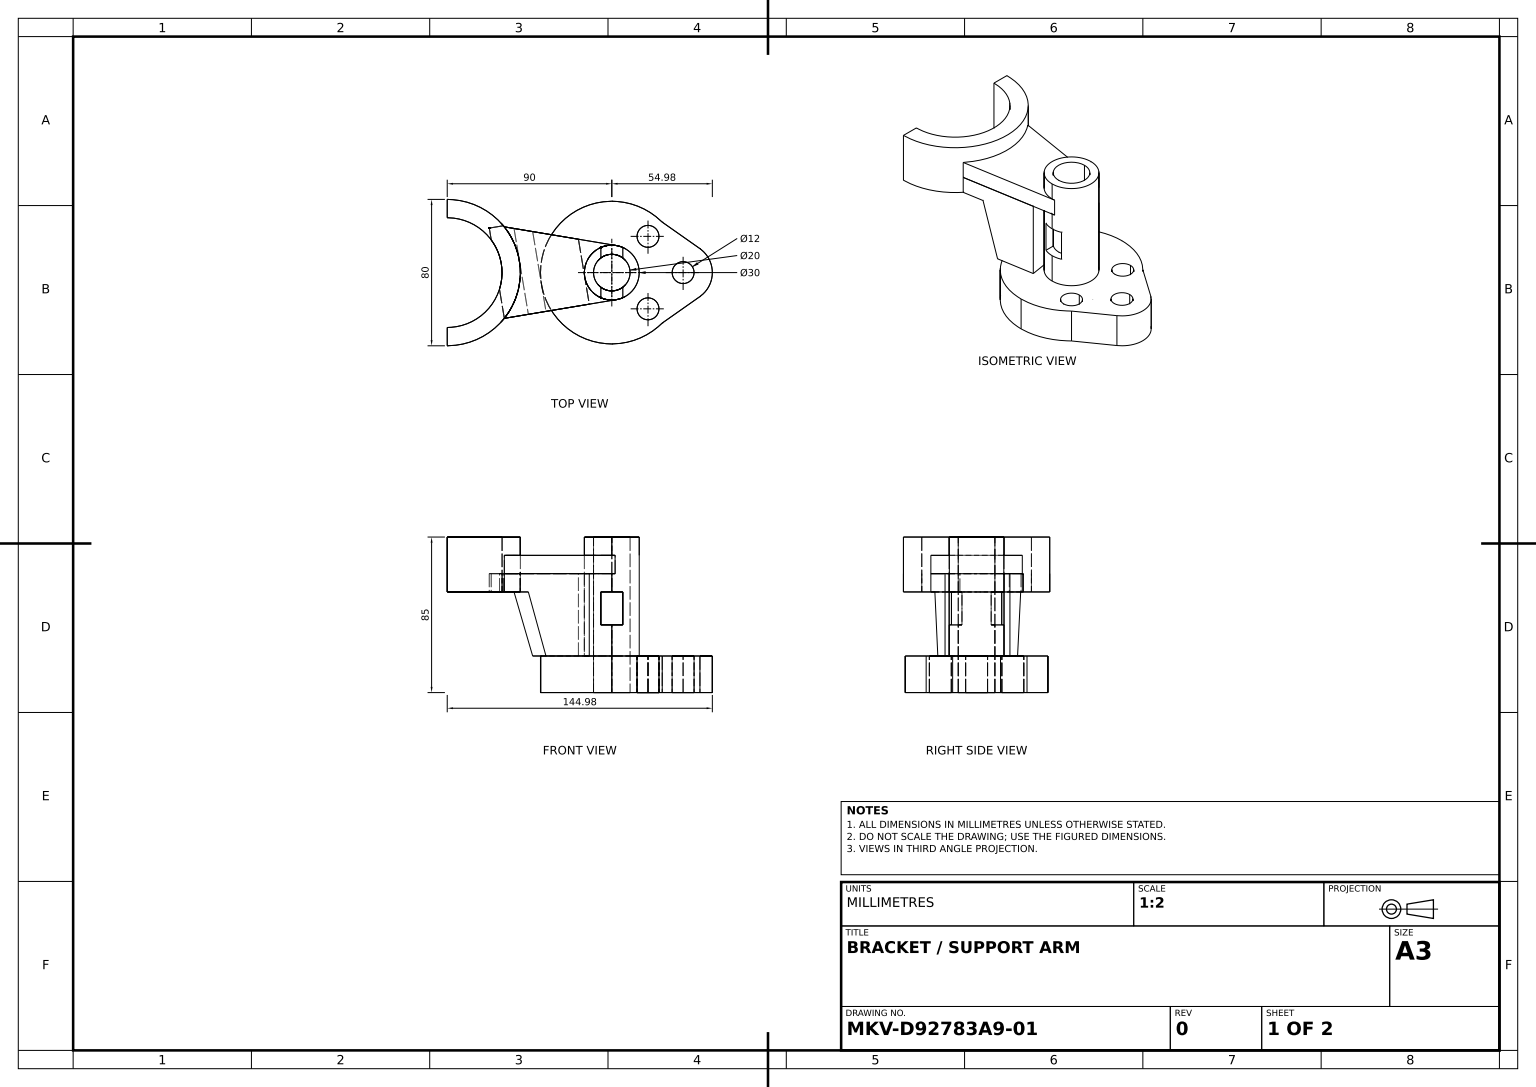
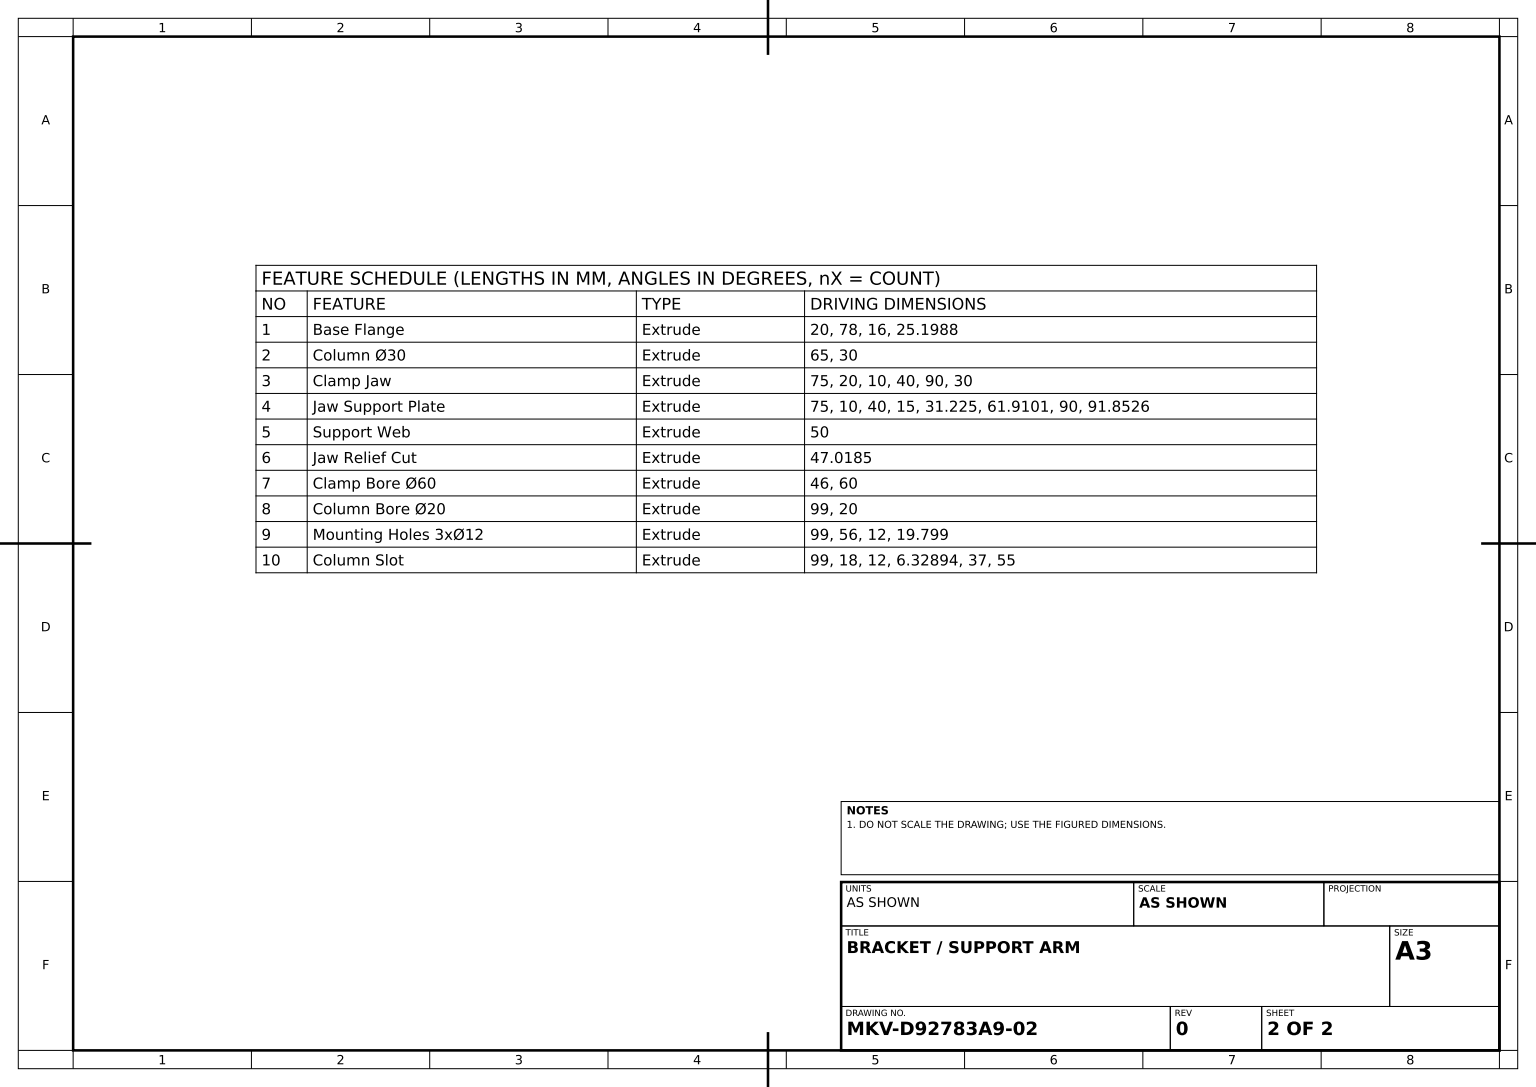
SolidWorks part; units mm, degrees
material "Plain Carbon Steel"
ref_plane "Front Plane" through (0, 0, 0) normal (0, 0, 1) x (1, 0, 0)
ref_plane "Top Plane" through (0, 0, 0) normal (0, 1, 0) x (1, 0, 0)
ref_plane "Right Plane" through (0, 0, 0) normal (1, 0, 0) x (0, 0, -1)
sketch "Base Flange Sketch" plane through (0, 0, 0) normal (0, 1, 0) x (1, 0, 0)
  line L2 (48.197, 13.0926) -> (27.5772, 27.5772)
  line L3 (27.5772, -27.5772) -> (48.197, -13.0926)
  arc A0 (27.5772, 27.5772) -> (27.5772, -27.5772) centre (0, 0) ccw
  arc A1 (48.197, -13.0926) -> (48.197, 13.0926) centre (39, 0) ccw
  dimension "D1" = 78
  dimension "D2" = 16
  dimension "D3" = 25.1988
  dimension "D4" = 25.1988
extrude "Base Flange" add sketch "Base Flange Sketch" along normal blind 20
sketch "Column Sketch" plane through (0, 20, 0) normal (0, 1, 0) x (1, 0, 0)
  circle A0 centre (0, 0) radius 15
  dimension "D1" = 30
extrude "Column Ø30" add sketch "Column Sketch" along normal blind 65
ref_plane "Jaw Plane" through (0, 75, 0) normal (0, 1, 0) x (1, 0, 0)
sketch "Clamp Jaw Sketch" plane through (0, 75, 0) normal (0, 1, 0) x (1, 0, 0)
  line L1 (-90, 30) -> (-90, 40)
  line L2 (-90, -30) -> (-90, -40)
  arc A0 (-90, -40) -> (-90, 40) centre (-90, 0) ccw
  arc A1 (-90, -30) -> (-90, 30) centre (-90, 0) ccw
  dimension "D1" = 40
  dimension "D3" = 30
  dimension "D2" = 90
extrude "Clamp Jaw" add sketch "Clamp Jaw Sketch" against normal blind 20 and the other way blind 10 separate body
sketch "Jaw Support Plate Sketch" plane through (0, 75, 0) normal (0, 1, 0) x (1, 0, 0)
  line L1 (-90, 0) -> (-90, 25)
  line L2 (-90, 0) -> (-90, -25)
  line L3 (-90, 25) -> (-58.775, 25)
  line L4 (-58.775, 25) -> (1.8526, 14.8852)
  line L5 (-90, -25) -> (-58.775, -25)
  line L6 (-58.775, -25) -> (3.1351, -14.6687)
  arc A0 (1.7979, -14.8919) -> (3.1351, -14.6687) centre (0, 0) ccw
  arc A2 (-58.775, -25) -> (-58.775, 25) centre (-90, 0) ccw
  arc A3 (1.8526, 14.8852) -> (3.1351, -14.6687) centre (0, 0) ccw
  dimension "D1" = 40
  dimension "D2" = 15
  dimension "D3" = 31.225
  dimension "D4" = 61.9101
  dimension "D5" = 90
  dimension "D6" = 91.8526
extrude "Jaw Support Plate" add sketch "Jaw Support Plate Sketch" against normal blind 10 contours A3 L4 A2 L6
sketch "Support Web Sketch" plane through (2.4665, 0, 14.7803) normal (0.1646, 0, 0.9864) x (0.9864, 0, -0.1646)
  line L3 (-15, 65) -> (-15, 20)
  line L4 (-15, 20) -> (-39, 20)
  line L6 (-39, 20) -> (-48.7724, 55)
  line L7 (-62.0883, 65) -> (-62.0883, 55)
  line L8 (-62.0883, 55) -> (-48.7724, 55)
  line L10 (44, 75) -> (-44, 75) construction
  line L11 (-62.0883, 65) -> (-62.0883, 75) construction
  line L12 (-62.0883, 75) -> (-48.7724, 75)
  line L14 (-15, 65) -> (-62.0883, 65)
  line M3 (-62.0883, 65) -> (-0.6779, 65)
extrude "Support Web" add sketch "Support Web Sketch" against normal blind 50 separate body contours L7 L8 L6 L4 L3 M3
sketch "Jaw Relief Cut Sketch" plane through (0, 65, 0) normal (0, 1, 0) x (1, 0, 0)
  line L0 (-58.775, 25) -> (-18.2511, 18.2392)
  line L1 (-58.775, 25) -> (1.8526, 14.8852) construction
  line L2 (-20.5589, 32.0687) -> (-12.3289, -17.2493) construction
  line L3 (-18.2511, 18.2392) -> (-20.5589, 32.0687)
  line L4 (-20.5589, 32.0687) -> (-59.3474, 25.5959)
  line L5 (-67.005, 24.318) -> (-20.5589, 32.0687) construction
  arc A0 (-90, -40) -> (-90, 40) centre (-90, 0) ccw construction
  arc A1 (-58.775, -25) -> (-58.775, 25) centre (-90, 0) ccw construction
  arc A2 (-58.775, 25) -> (-59.2721, 25.6085) centre (-90, 0) ccw
  line M2 (-12.3289, -17.2493) -> (-20.5589, 32.0687)
  line M3 (-20.5589, 32.0687) -> (-67.005, 24.318)
  dimension "D1" = 47.0185
extrude "Jaw Relief Cut" cut sketch "Jaw Relief Cut Sketch" against normal up to vertex contours A2 L0 M2 M3
sketch "Clamp Bore Sketch" plane through (0, 85, 0) normal (0, 1, 0) x (1, 0, 0)
  circle A0 centre (-90, 0) radius 30
  dimension "D1" = 60
extrude "Clamp Bore Ø60" cut sketch "Clamp Bore Sketch" against normal blind 46
sketch "Column Bore Sketch" plane through (0, 85, 0) normal (0, 1, 0) x (1, 0, 0)
  circle A0 centre (0, 0) radius 10
  dimension "D1" = 20
extrude "Column Bore Ø20" cut sketch "Column Bore Sketch" against normal blind 99
sketch "Mounting Holes Sketch" plane through (0, 20, 0) normal (0, 1, 0) x (1, 0, 0)
  circle A0 centre (39, 0) radius 6
  circle A1 centre (0, 0) radius 28 construction
  circle A2 centre (19.799, 19.799) radius 6
  circle A3 centre (19.799, -19.799) radius 6
  dimension "D1" = 56
  dimension "D2" = 12
  dimension "D3" = 12
  dimension "D4" = 12
  dimension "D5" = 19.799
  dimension "D6" = 19.799
extrude "Mounting Holes 3xØ12" cut sketch "Mounting Holes Sketch" against normal blind 99
sketch "Column Slot Sketch" plane through (0, 0, 0) normal (0, 0, 1) x (1, 0, 0)
  line L0 (-12.3289, 65) -> (-12.3289, 20) construction
  line L2 (0, 55) -> (6, 55)
  line L3 (6, 55) -> (6, 37)
  line L4 (6, 37) -> (-6, 37)
  line L5 (-6, 37) -> (-6, 55)
  line L6 (-6, 55) -> (0, 55)
  dimension "D1" = 18
  dimension "D2" = 12
  dimension "D3" = 6.3289
  dimension "D4" = 37
  dimension "D5" = 55
extrude "Column Slot" cut sketch "Column Slot Sketch" against normal mid plane 99
